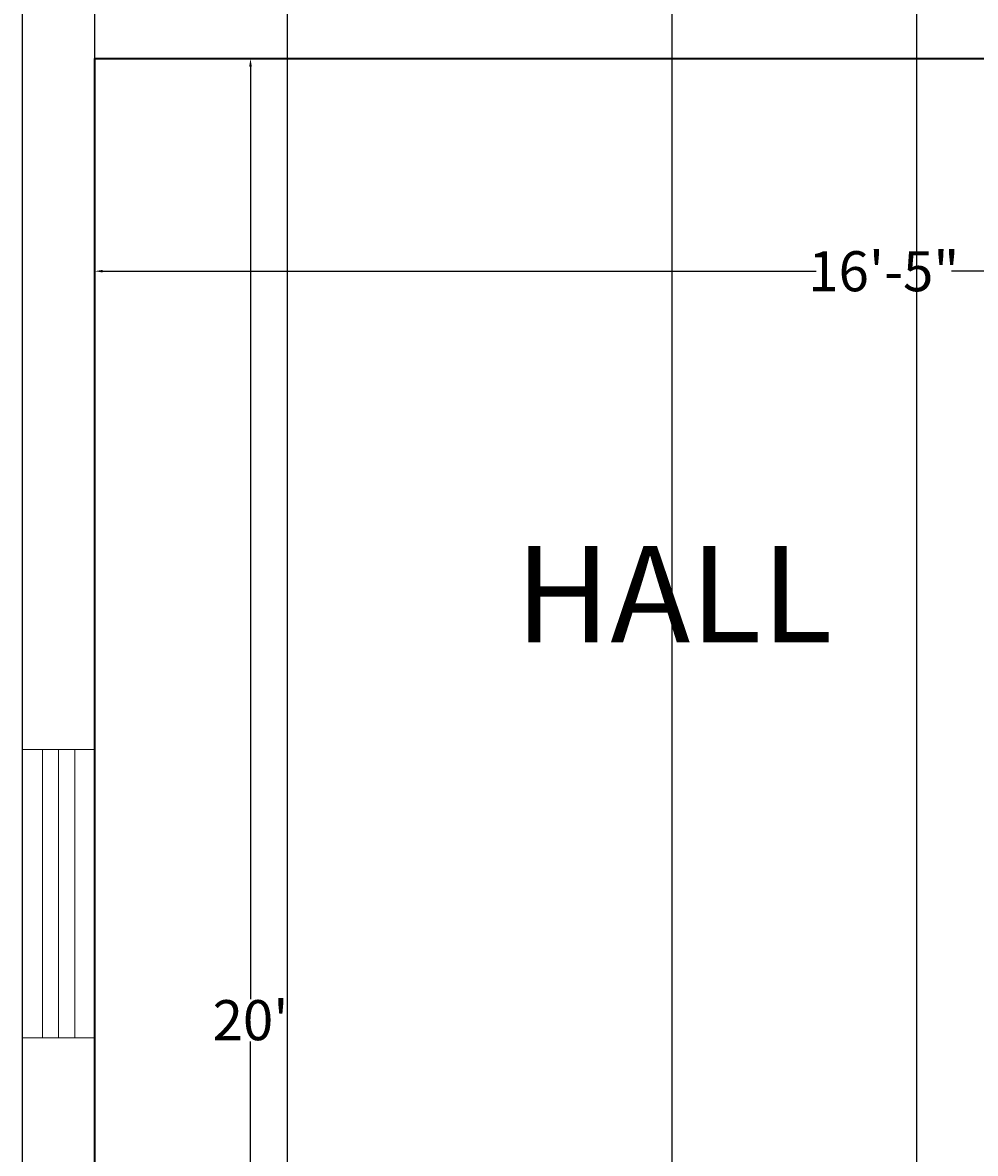
# Model space of a CAD drawing. Units: inches. Extents: x -304 to 580, y 363 to 1149.
# Tile 6 of 11: x -23 to 96, y 653 to 794. Entities that reach past the tile are written whole.
import ezdxf

# ---------------------------------------------------------------- set-up
doc = ezdxf.new("R2010")
doc.units = ezdxf.units.IN
doc.header["$MEASUREMENT"] = 0
for name, color, linetype, lineweight in [('A-ANNO-DIMS', 2, 'Continuous', 13), ('A-AREA-IDEN', 7, 'Continuous', 25), ('A-GLAZ', 4, 'Continuous', 18), ('A-WALL', 40, 'Continuous', 35)]:
    doc.layers.add(name, color=color, linetype=linetype, lineweight=lineweight)
doc.styles.get("Standard").update_dxf_attribs({"font": 'arial.ttf'})
doc.dimstyles.get("Standard").update_dxf_attribs({"dimtxt": 1, "dimasz": 1, "dimexe": 0.18, "dimexo": 0.0625, "dimgap": 0.09, "dimtad": 0, "dimtih": 1, "dimtoh": 1, "dimdec": 0, "dimzin": 0, "dimdsep": 46, "dimlunit": 3, "dimtxsty": 'Standard', "dimcen": 0.09, "dimadec": 0, "dimazin": 0, "dimtfac": 1, "dimtdec": 0, "dimtofl": 0, "dimtmove": 0, "dimatfit": 3, "dimfxl": 1, "dimtolj": 1, "dimtzin": 0, "dimarcsym": 0})

# ---------------------------------------------------------------- blocks, each defined once
blk = doc.blocks.new('*D3')
at = {"layer": 'A-ANNO-DIMS', "color": 0, "lineweight": -2, "transparency": 16777216}
for p, q in [((-13.51, 789.95), (6.06, 789.95)), ((5.88, 788.95), (5.88, 672.59)), ((5.88, 550.95), (5.88, 667.3)), ((-13.51, 549.95), (6.06, 549.95))]:
    blk.add_line(p, q, dxfattribs=at)
at = {"layer": 'A-ANNO-DIMS', "color": 0, "transparency": 16777216}
for points in [[(5.71, 788.95), (6.04, 788.95), (5.88, 789.95)], [(5.71, 550.95), (6.04, 550.95), (5.88, 549.95)]]:
    blk.add_solid(points, dxfattribs=at)
at = {"layer": 'Defpoints', "color": 0, "transparency": 16777216}
for p in [(-13.57, 789.95), (5.88, 789.95), (-13.57, 549.95)]:
    blk.add_point(p, dxfattribs=at)
at = {"layer": 'A-ANNO-DIMS', "color": 0, "transparency": 16777216, "insert": (5.88, 669.95), "char_height": 1, "attachment_point": 5}
blk.add_mtext("\\A1;{\\H5x;20'}", dxfattribs=at)
blk = doc.blocks.new('*D4')
at = {"layer": 'A-ANNO-DIMS', "color": 0, "lineweight": -2, "transparency": 16777216}
for p, q in [((-13.57, 789.88), (-13.57, 763.24)), ((183.43, 789.88), (183.43, 763.24)), ((-12.57, 763.42), (76.49, 763.42)), ((182.43, 763.42), (93.37, 763.42))]:
    blk.add_line(p, q, dxfattribs=at)
at = {"layer": 'A-ANNO-DIMS', "color": 0, "transparency": 16777216}
for points in [[(-12.57, 763.59), (-12.57, 763.26), (-13.57, 763.42)], [(182.43, 763.59), (182.43, 763.26), (183.43, 763.42)]]:
    blk.add_solid(points, dxfattribs=at)
at = {"layer": 'Defpoints', "color": 0, "transparency": 16777216}
for p in [(-13.57, 789.95), (183.43, 789.95), (183.43, 763.42)]:
    blk.add_point(p, dxfattribs=at)
at = {"layer": 'A-ANNO-DIMS', "color": 0, "transparency": 16777216, "insert": (84.93, 763.42), "char_height": 1, "attachment_point": 5}
blk.add_mtext('\\A1;{\\H5x;16\'-5"}', dxfattribs=at)
blk = doc.blocks.new('WIN-36IN')
for p, q in [((0, 6.5), (36, 6.5)), ((0, 4.5), (36, 4.5)), ((0, 2.5), (36, 2.5))]:
    blk.add_line(p, q)
blk.add_lwpolyline([(0, 0), (0, 9), (36, 9), (36, 0)], close=True)
blk = doc.blocks.new('*D34')
at = {"layer": 'A-ANNO-DIMS', "color": 0, "lineweight": -2, "transparency": 16777216}
for p, q in [((10.51, 550.01), (10.51, 1042.88)), ((11.51, 1042.7), (33.07, 1042.7)), ((57.51, 1042.7), (35.95, 1042.7)), ((58.51, 550.01), (58.51, 1042.88))]:
    blk.add_line(p, q, dxfattribs=at)
at = {"layer": 'A-ANNO-DIMS', "color": 0, "transparency": 16777216}
for points in [[(11.51, 1042.86), (11.51, 1042.53), (10.51, 1042.7)], [(57.51, 1042.86), (57.51, 1042.53), (58.51, 1042.7)]]:
    blk.add_solid(points, dxfattribs=at)
at = {"layer": 'Defpoints', "color": 0, "transparency": 16777216}
for p in [(58.51, 1042.7), (10.51, 549.95), (58.51, 549.95)]:
    blk.add_point(p, dxfattribs=at)
at = {"layer": 'A-ANNO-DIMS', "color": 0, "transparency": 16777216, "insert": (34.51, 1042.7), "char_height": 1, "attachment_point": 5}
blk.add_mtext('\\A1;4\'-0"', dxfattribs=at)
blk = doc.blocks.new('*D35')
at = {"layer": 'A-ANNO-DIMS', "color": 0, "lineweight": -2, "transparency": 16777216}
for p, q in [((-13.57, 550.01), (-13.57, 1042.88)), ((-12.57, 1042.7), (-2.96, 1042.7)), ((9.51, 1042.7), (-0.1, 1042.7)), ((10.51, 550.01), (10.51, 1042.88))]:
    blk.add_line(p, q, dxfattribs=at)
at = {"layer": 'A-ANNO-DIMS', "color": 0, "transparency": 16777216}
for points in [[(-12.57, 1042.86), (-12.57, 1042.53), (-13.57, 1042.7)], [(9.51, 1042.86), (9.51, 1042.53), (10.51, 1042.7)]]:
    blk.add_solid(points, dxfattribs=at)
at = {"layer": 'Defpoints', "color": 0, "transparency": 16777216}
for p in [(10.51, 1042.7), (-13.57, 549.95), (10.51, 549.95)]:
    blk.add_point(p, dxfattribs=at)
at = {"layer": 'A-ANNO-DIMS', "color": 0, "transparency": 16777216, "insert": (-1.53, 1042.7), "char_height": 1, "attachment_point": 5}
blk.add_mtext('\\A1;2\'-0"', dxfattribs=at)
blk = doc.blocks.new('*D36')
at = {"layer": 'A-ANNO-DIMS', "color": 0, "lineweight": -2, "transparency": 16777216}
for p, q in [((-22.57, 516.57), (-22.57, 1042.88)), ((-21.57, 1042.7), (30.65, 1042.7)), ((88.04, 1042.7), (35.82, 1042.7)), ((89.04, 516.57), (89.04, 1042.88))]:
    blk.add_line(p, q, dxfattribs=at)
at = {"layer": 'A-ANNO-DIMS', "color": 0, "transparency": 16777216}
for points in [[(-21.57, 1042.86), (-21.57, 1042.53), (-22.57, 1042.7)], [(88.04, 1042.86), (88.04, 1042.53), (89.04, 1042.7)]]:
    blk.add_solid(points, dxfattribs=at)
at = {"layer": 'Defpoints', "color": 0, "transparency": 16777216}
for p in [(89.04, 1042.7), (-22.57, 516.51), (89.04, 516.51)]:
    blk.add_point(p, dxfattribs=at)
at = {"layer": 'A-ANNO-DIMS', "color": 0, "transparency": 16777216, "insert": (33.23, 1042.7), "char_height": 1, "attachment_point": 5}
blk.add_mtext('\\A1;9\'-3 1/2"', dxfattribs=at)

msp = doc.modelspace()

# ---------------------------------------------------------------- linework, layer by layer
at = {"layer": 'A-WALL'}
for p, q in [((-13.57, 789.95), (111.43, 789.95)), ((-13.57, 549.95), (-13.57, 789.95))]:
    msp.add_line(p, q, dxfattribs=at)

# ---------------------------------------------------------------- block references
at = {"layer": 'A-GLAZ', "rotation": 270.0000000000002}
msp.add_blockref('WIN-36IN', (-22.57, 703.75), dxfattribs=at)

# ---------------------------------------------------------------- texts
at = {"layer": 'A-AREA-IDEN', "insert": (38.89, 729.12), "char_height": 12, "attachment_point": 1}
msp.add_mtext_dynamic_manual_height_columns('HALL', width=65.0856, gutter_width=1, heights=[0], dxfattribs=at)

# ---------------------------------------------------------------- dimensions: what is measured, and where the dimension line sits
at = {"layer": 'A-ANNO-DIMS'}
for base, p1, p2, picture, middle in [((89.04, 1042.7), (-22.57, 516.51), (89.04, 516.51), '*D36', (33.23, 1042.7)), ((10.51, 1042.7), (-13.57, 549.95), (10.51, 549.95), '*D35', (-1.53, 1042.7)), ((58.51, 1042.7), (10.51, 549.95), (58.51, 549.95), '*D34', (34.51, 1042.7))]:
    dim = msp.add_linear_dim(base=base, p1=p1, p2=p2, dimstyle='Standard', override={"dimdec": 1, "dimlfac": 1, "dimrnd": 0, "dimzin": 1, "dimdsep": 46, "dimlunit": 4, "dimfrac": 2}, dxfattribs=at)
    dim.commit()
    dim.dimension.update_dxf_attribs({"geometry": picture, "text_midpoint": middle})
dim = msp.add_linear_dim(base=(5.88, 789.95), p1=(-13.57, 549.95), p2=(-13.57, 789.95), angle=90, text='{\\H5x;<>}', dimstyle='Standard', override={"dimclrd": 0, "dimclre": 0, "dimclrt": 0}, dxfattribs=at)
dim.commit()
dim.dimension.update_dxf_attribs({"geometry": '*D3', "text_midpoint": (5.88, 669.95)})
dim = msp.add_linear_dim(base=(183.43, 763.42), p1=(-13.57, 789.95), p2=(183.43, 789.95), text='{\\H5x;<>}', dimstyle='Standard', override={"dimclrd": 0, "dimclre": 0, "dimclrt": 0}, dxfattribs=at)
dim.commit()
dim.dimension.update_dxf_attribs({"geometry": '*D4', "text_midpoint": (84.93, 763.42)})

doc.saveas('drawing.dxf')
